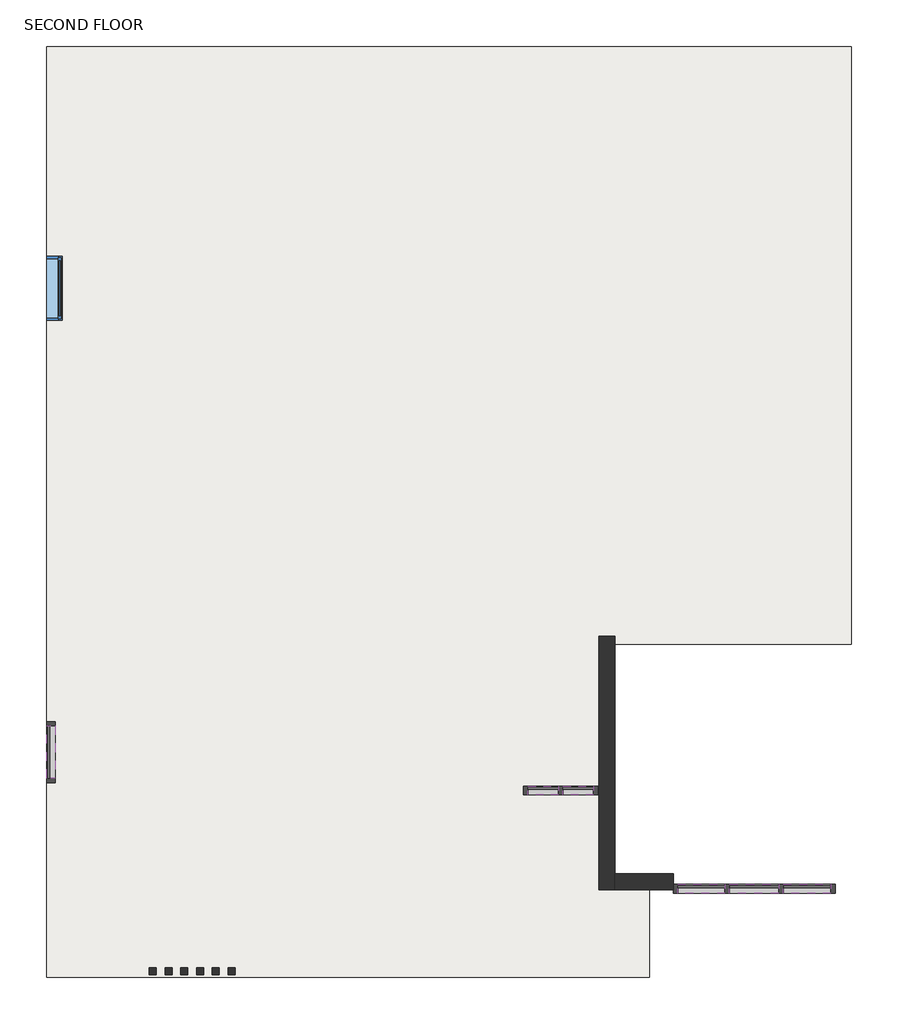
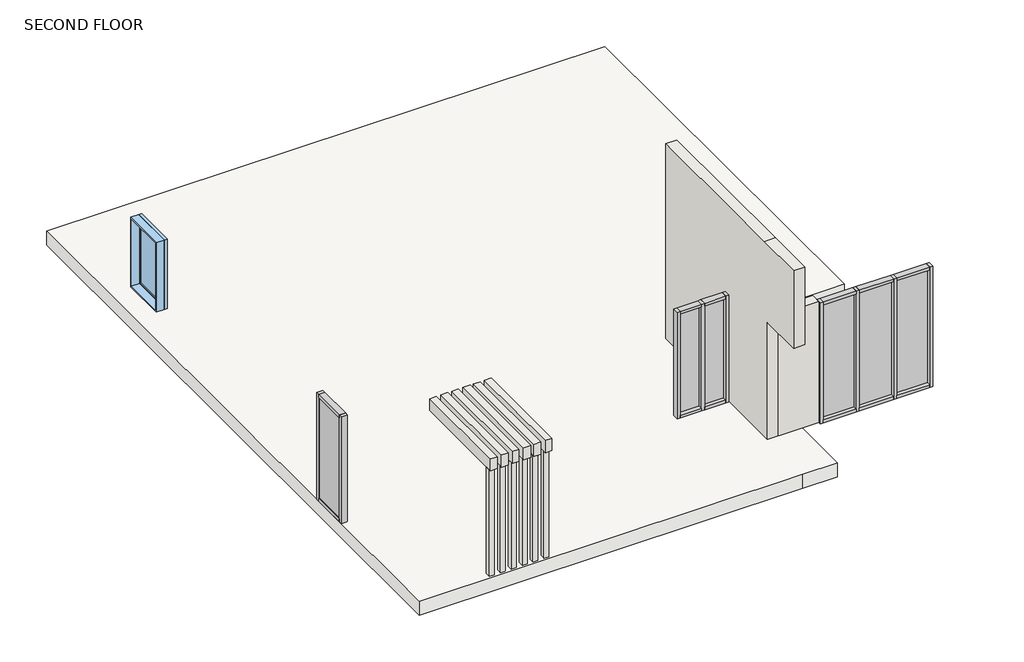
# One storey, incomplete: 21 members, 6 plates, 3 walls, 1 slab, 1 window.
"""IFC4 building model written with IfcOpenShell, lengths in millimetres."""

from ifc_helpers import new_model, si_unit, frame, origin, place, context, project, spatial, polyline, outline, extrude, faceted_brep, transform, mapped, element, save
from components import member_9bbf3b0c, member_f77fa896, member_3f28283e, member_3cbf331d, member_1631f5ff, member_7823a6e7, member_6fb4a552, member_def95f85, system_panel_glazed_aa1e9ff3, system_panel_glazed_6ccdd28e, system_panel_glazed_5a379f96, system_panel_glazed_6abed3b5, walls_2_walls_2_a9f40376, window_cd393ee1

model = new_model("IFC4")

# Units and contexts
model_context = context("Model", 3, world=origin())
ifc_project = project(units=[si_unit("LENGTHUNIT", "METRE", prefix="MILLI")], contexts=[model_context])

# Site, building, storey
site = spatial("IfcSite", under=ifc_project)
building = spatial("IfcBuilding", under=site)
storey = spatial("IfcBuildingStorey", under=building, Name="SECOND FLOOR", Elevation=6096.0)

# Members
placement = place(None, origin())
member_shape = member_9bbf3b0c(model_context)
element("IfcMember", 1, ObjectType="Rectangular Mullion : 2.5\" x 5\" rectangular", at=placement, inside=storey, context=model_context, shape_type="MappedRepresentation", body=[
    mapped(member_shape, transform((94.5792748, 2415.8467494, 6096.0), x_axis=(1.0, 0.0, 0.0), y_axis=(0.0, -1.0, 0.0), z_axis=(0.0, 0.0, -1.0))),
])
element("IfcMember", 2, ObjectType="Rectangular Mullion : 2.5\" x 5\" rectangular", at=placement, inside=storey, context=model_context, shape_type="MappedRepresentation", body=[
    mapped(member_shape, transform((-7754.0425919, 3404.9615229, 6096.0), x_axis=(0.0, 1.0, 0.0), y_axis=(1.0, 0.0, 0.0), z_axis=(0.0, 0.0, -1.0))),
])
element("IfcMember", 3, ObjectType="Rectangular Mullion : 2.5\" x 5\" rectangular", at=placement, inside=storey, context=model_context, shape_type="MappedRepresentation", body=[
    mapped(member_shape, transform((-972.2207252, 2415.8467494, 8432.8), x_axis=(-1.0, 0.0, 0.0), y_axis=(0.0, -1.0, 0.0), z_axis=(0.0, 0.0, 1.0))),
])
element("IfcMember", 4, ObjectType="Rectangular Mullion : 2.5\" x 5\" rectangular", at=placement, inside=storey, context=model_context, shape_type="MappedRepresentation", body=[
    mapped(member_shape, transform((-7754.0425919, 2530.1467494, 8432.8), x_axis=(0.0, -1.0, 0.0), y_axis=(1.0, 0.0, 0.0), z_axis=(0.0, 0.0, 1.0))),
])
member_2_shape = member_f77fa896(model_context)
element("IfcMember", 5, ObjectType="Rectangular Mullion : 2.5\" x 5\" rectangular", at=placement, inside=storey, context=model_context, shape_type="MappedRepresentation", body=[
    mapped(member_2_shape, transform((-7754.0425919, 3341.4615229, 8432.8), x_axis=(0.0, 0.0, 1.0), y_axis=(1.0, 0.0, 0.0), z_axis=(0.0, 1.0, 0.0))),
])
element("IfcMember", 6, ObjectType="Rectangular Mullion : 2.5\" x 5\" rectangular", at=placement, inside=storey, context=model_context, shape_type="MappedRepresentation", body=[
    mapped(member_2_shape, transform((-7754.0425919, 2593.6467494, 6096.0), x_axis=(0.0, 0.0, -1.0), y_axis=(1.0, 0.0, 0.0), z_axis=(0.0, -1.0, 0.0))),
])
member_3_shape = member_3f28283e(model_context)
element("IfcMember", 7, ObjectType="Rectangular Mullion : 2.5\" x 5\" rectangular", at=placement, inside=storey, context=model_context, shape_type="MappedRepresentation", body=[
    mapped(member_3_shape, transform((3498.0918749, 1006.1953049, 6096.0), x_axis=(1.0, 0.0, 0.0), y_axis=(0.0, -1.0, 0.0), z_axis=(0.0, 0.0, -1.0))),
])
element("IfcMember", 8, ObjectType="Rectangular Mullion : 2.5\" x 5\" rectangular", at=placement, inside=storey, context=model_context, shape_type="MappedRepresentation", body=[
    mapped(member_3_shape, transform((1173.991862, 1006.1953049, 8737.6), x_axis=(-1.0, 0.0, 0.0), y_axis=(0.0, -1.0, 0.0), z_axis=(0.0, 0.0, 1.0))),
])
member_4_shape = member_3cbf331d(model_context)
element("IfcMember", 9, ObjectType="Rectangular Mullion : 2.5\" x 5\" rectangular", at=placement, inside=storey, context=model_context, shape_type="MappedRepresentation", body=[
    mapped(member_4_shape, transform((1237.491862, 1006.1953049, 6096.0), x_axis=(0.0, 0.0, -1.0), y_axis=(0.0, -1.0, 0.0), z_axis=(-1.0, 0.0, 0.0))),
])
element("IfcMember", 10, ObjectType="Rectangular Mullion : 2.5\" x 5\" rectangular", at=placement, inside=storey, context=model_context, shape_type="MappedRepresentation", body=[
    mapped(member_4_shape, transform((2755.1418706, 1006.1953049, 6096.0), x_axis=(0.0, 0.0, -1.0), y_axis=(0.0, -1.0, 0.0), z_axis=(-1.0, 0.0, 0.0))),
])
element("IfcMember", 11, ObjectType="Rectangular Mullion : 2.5\" x 5\" rectangular", at=placement, inside=storey, context=model_context, shape_type="MappedRepresentation", body=[
    mapped(member_4_shape, transform((3434.5918749, 1006.1953049, 8737.6), x_axis=(0.0, 0.0, 1.0), y_axis=(0.0, -1.0, 0.0), z_axis=(1.0, 0.0, 0.0))),
])
element("IfcMember", 12, ObjectType="Rectangular Mullion : 2.5\" x 5\" rectangular", at=placement, inside=storey, context=model_context, shape_type="MappedRepresentation", body=[
    mapped(member_4_shape, transform((1916.9418663, 1006.1953049, 8737.6), x_axis=(0.0, 0.0, 1.0), y_axis=(0.0, -1.0, 0.0), z_axis=(1.0, 0.0, 0.0))),
])
member_5_shape = member_1631f5ff(model_context)
element("IfcMember", 13, ObjectType="Rectangular Mullion : 2.5\" x 5\" rectangular", at=placement, inside=storey, context=model_context, shape_type="MappedRepresentation", body=[
    mapped(member_5_shape, transform((1948.6918663, 1006.1953049, 6096.0), x_axis=(1.0, 0.0, 0.0), y_axis=(0.0, -1.0, 0.0), z_axis=(0.0, 0.0, -1.0))),
])
element("IfcMember", 14, ObjectType="Rectangular Mullion : 2.5\" x 5\" rectangular", at=placement, inside=storey, context=model_context, shape_type="MappedRepresentation", body=[
    mapped(member_5_shape, transform((2723.3918706, 1006.1953049, 6096.0), x_axis=(1.0, 0.0, 0.0), y_axis=(0.0, -1.0, 0.0), z_axis=(0.0, 0.0, -1.0))),
])
member_6_shape = member_7823a6e7(model_context)
element("IfcMember", 15, ObjectType="Rectangular Mullion : 2.5\" x 5\" rectangular", at=placement, inside=storey, context=model_context, shape_type="MappedRepresentation", body=[
    mapped(member_6_shape, transform((1980.4418663, 1006.1953049, 6096.0), x_axis=(0.0, 0.0, -1.0), y_axis=(0.0, -1.0, 0.0), z_axis=(-1.0, 0.0, 0.0))),
])
element("IfcMember", 16, ObjectType="Rectangular Mullion : 2.5\" x 5\" rectangular", at=placement, inside=storey, context=model_context, shape_type="MappedRepresentation", body=[
    mapped(member_6_shape, transform((2691.6418706, 1006.1953049, 8737.6), x_axis=(0.0, 0.0, 1.0), y_axis=(0.0, -1.0, 0.0), z_axis=(1.0, 0.0, 0.0))),
])
member_7_shape = member_6fb4a552(model_context)
element("IfcMember", 17, ObjectType="Rectangular Mullion : 2.5\" x 5\" rectangular", at=placement, inside=storey, context=model_context, shape_type="MappedRepresentation", body=[
    mapped(member_7_shape, transform((31.0792748, 2415.8467494, 8432.8), x_axis=(0.0, 0.0, 1.0), y_axis=(0.0, -1.0, 0.0), z_axis=(1.0, 0.0, 0.0))),
])
element("IfcMember", 18, ObjectType="Rectangular Mullion : 2.5\" x 5\" rectangular", at=placement, inside=storey, context=model_context, shape_type="MappedRepresentation", body=[
    mapped(member_7_shape, transform((-470.5707252, 2415.8467494, 8432.8), x_axis=(0.0, 0.0, 1.0), y_axis=(0.0, -1.0, 0.0), z_axis=(1.0, 0.0, 0.0))),
])
element("IfcMember", 19, ObjectType="Rectangular Mullion : 2.5\" x 5\" rectangular", at=placement, inside=storey, context=model_context, shape_type="MappedRepresentation", body=[
    mapped(member_7_shape, transform((-908.7207252, 2415.8467494, 6096.0), x_axis=(0.0, 0.0, -1.0), y_axis=(0.0, -1.0, 0.0), z_axis=(-1.0, 0.0, 0.0))),
])
element("IfcMember", 20, ObjectType="Rectangular Mullion : 2.5\" x 5\" rectangular", at=placement, inside=storey, context=model_context, shape_type="MappedRepresentation", body=[
    mapped(member_7_shape, transform((-407.0707252, 2415.8467494, 6096.0), x_axis=(0.0, 0.0, -1.0), y_axis=(0.0, -1.0, 0.0), z_axis=(-1.0, 0.0, 0.0))),
])
member_8_shape = member_def95f85(model_context)
element("IfcMember", 21, ObjectType="Rectangular Mullion : 2.5\" x 5\" rectangular", at=placement, inside=storey, context=model_context, shape_type="MappedRepresentation", body=[
    mapped(member_8_shape, transform((-438.8207252, 2415.8467494, 6096.0), x_axis=(1.0, 0.0, 0.0), y_axis=(0.0, -1.0, 0.0), z_axis=(0.0, 0.0, -1.0))),
])

# Plates
system_panel_glazed_shape = system_panel_glazed_aa1e9ff3(model_context)
element("IfcPlate", 22, ObjectType="System Panel : Glazed", at=placement, inside=storey, context=model_context, shape_type="MappedRepresentation", body=[
    mapped(system_panel_glazed_shape, transform((-7754.0425919, 2967.5541361, 6159.5), x_axis=(0.0, 1.0, 0.0), y_axis=(-1.0, 0.0, 0.0), z_axis=(0.0, 0.0, 1.0))),
])
system_panel_glazed_2_shape = system_panel_glazed_6ccdd28e(model_context)
element("IfcPlate", 23, ObjectType="System Panel : Glazed", at=placement, inside=storey, context=model_context, shape_type="MappedRepresentation", body=[
    mapped(system_panel_glazed_2_shape, transform((1577.2168642, 1006.1953049, 6159.5), x_axis=(1.0, 0.0, 0.0), y_axis=(0.0, 1.0, 0.0), z_axis=(0.0, 0.0, 1.0))),
])
element("IfcPlate", 24, ObjectType="System Panel : Glazed", at=placement, inside=storey, context=model_context, shape_type="MappedRepresentation", body=[
    mapped(system_panel_glazed_2_shape, transform((3094.8668728, 1006.1953049, 6159.5), x_axis=(1.0, 0.0, 0.0), y_axis=(0.0, 1.0, 0.0), z_axis=(0.0, 0.0, 1.0))),
])
system_panel_glazed_3_shape = system_panel_glazed_5a379f96(model_context)
element("IfcPlate", 25, ObjectType="System Panel : Glazed", at=placement, inside=storey, context=model_context, shape_type="MappedRepresentation", body=[
    mapped(system_panel_glazed_3_shape, transform((2336.0418685, 1006.1953049, 6159.5), x_axis=(1.0, 0.0, 0.0), y_axis=(0.0, 1.0, 0.0), z_axis=(0.0, 0.0, 1.0))),
])
system_panel_glazed_4_shape = system_panel_glazed_6abed3b5(model_context)
element("IfcPlate", 26, ObjectType="System Panel : Glazed", at=placement, inside=storey, context=model_context, shape_type="MappedRepresentation", body=[
    mapped(system_panel_glazed_4_shape, transform((-689.6457252, 2415.8467494, 6159.5), x_axis=(1.0, 0.0, 0.0), y_axis=(0.0, 1.0, 0.0), z_axis=(0.0, 0.0, 1.0))),
])
element("IfcPlate", 27, ObjectType="System Panel : Glazed", at=placement, inside=storey, context=model_context, shape_type="MappedRepresentation", body=[
    mapped(system_panel_glazed_4_shape, transform((-187.9957252, 2415.8467494, 6159.5), x_axis=(1.0, 0.0, 0.0), y_axis=(0.0, 1.0, 0.0), z_axis=(0.0, 0.0, 1.0))),
])

# Slab
element("IfcSlab", 28, ObjectType="Generic - 12\"", at=placement, inside=storey, context=model_context, shape_type="SweptSolid", body=[
    extrude(outline(polyline([(3726.6918749, 13083.8953049), (3726.6918749, 4511.3953049), (107.1918749, 4511.3953049), (107.1918749, 993.4953049), (831.1355684, 993.4953049), (831.1355684, -263.8046951), (108.6382856, -263.8046951), (-7817.6081251, -263.8046951), (-7817.6081251, 13083.8953049), (3726.6918749, 13083.8953049)])), frame((0.0, 0.0, 5791.2), z_axis=(0.0, 0.0, 1.0), x_axis=(1.0, 0.0, 0.0)), (0.0, 0.0, 1.0), 304.8),
])

# Walls
element("IfcWall", 29, ObjectType="9\"", at=placement, inside=storey, context=model_context, shape_type="Brep", body=[
    faceted_brep([(335.8792748, 993.4953049, 6096.0), (335.8792748, 1222.0953049, 6096.0), (335.8792748, 4625.6953049, 6096.0), (335.8792748, 4625.6953049, 10363.2), (335.8792748, 1107.7953049, 10363.2), (335.8792748, 282.2953049, 10363.2), (335.8792748, 53.6953049, 10363.2), (335.8792748, 53.6953049, 8737.6), (335.8792748, 53.6953049, 8661.4), (335.8792748, 993.4953049, 8661.4), (107.2792748, 993.4953049, 6096.0), (107.2792748, 993.4953049, 8661.4), (107.2792748, 53.6953049, 8661.4), (107.2792748, 53.6953049, 10363.2), (107.2792748, 1107.7953049, 10363.2), (107.2792748, 1895.1953049, 10363.2), (107.2792748, 2123.7953049, 10363.2), (107.2792748, 4625.6953049, 10363.2), (107.2792748, 4625.6953049, 6096.0)], [[[0, 1, 2, 3, 4, 5, 6, 7, 8, 9]], [[10, 11, 12, 13, 14, 15, 16, 17, 18]], [[2, 1, 0, 10, 18]], [[3, 2, 18, 17]], [[4, 3, 17, 16, 15, 14]], [[6, 5, 4, 14, 13]], [[8, 7, 6, 13, 12]], [[9, 8, 12, 11]], [[0, 9, 11, 10]]]),
])
element("IfcWall", 30, ObjectType="9\"", at=placement, inside=storey, context=model_context, shape_type="Brep", body=[
    faceted_brep([(335.8792748, 993.4953049, 8737.6), (335.8792748, 993.4953049, 8661.4), (335.8792748, 993.4953049, 6096.0), (1173.991862, 993.4953049, 6096.0), (1173.991862, 993.4953049, 8737.6), (335.8792748, 1222.0953049, 6096.0), (335.8792748, 1222.0953049, 8737.6), (1173.991862, 1222.0953049, 8737.6), (1173.991862, 1222.0953049, 6096.0)], [[[0, 1, 2, 3, 4]], [[5, 6, 7, 8]], [[3, 2, 5, 8]], [[4, 3, 8, 7]], [[0, 4, 7, 6]], [[0, 6, 5, 2, 1]]]),
])
walls_2_walls_2_shape = walls_2_walls_2_a9f40376(model_context)
element("IfcWall", 31, ObjectType="Walls 2 : Walls 2", at=placement, inside=storey, context=model_context, shape_type="MappedRepresentation", body=[
    mapped(walls_2_walls_2_shape, transform((0.0, 0.0, 0.0), x_axis=(1.0, 0.0, 0.0), y_axis=(0.0, 1.0, 0.0), z_axis=(0.0, 0.0, 1.0))),
])

# Window
window_shape = window_cd393ee1(model_context)
element("IfcWindow", 32, ObjectType="Fixed : 36\" x 48\"", at=placement, inside=storey, context=model_context, shape_type="MappedRepresentation", body=[
    mapped(window_shape, transform((-7703.3081251, 9578.6953049, 5791.2), x_axis=(0.0, -1.0, 0.0), y_axis=(1.0, 0.0, 0.0), z_axis=(0.0, 0.0, 1.0))),
])

save(model, "model.ifc")

# Revit data of these elements
# Type "Rectangular Mullion : 2.5\" x 5\" rectangular"
#   built-in parameter 1007304 = 0.416667 (stored number, unit not read)
#   built-in parameter 1007301 = 0.104167 (stored number, unit not read)
#   built-in parameter 1007300 = 0.104167 (stored number, unit not read)
# Type "System Panel : Glazed"
#   Construction Type Id = "GSP4R"
#   Analytic Construction = "1/8 in Pilkington single glazing"
#   Visual Light Transmittance = 0.9
#   Solar Heat Gain Coefficient = 0.86
#   Heat Transfer Coefficient (U) = 1.18115 BTU/(h·ft²·°F)
#   Define Thermal Properties by = 1
# Type "Generic - 12\""
#   Assembly Code = "B1010"
#   Function = 0
#   Layers, outside or top first: 1' - 0" no material (function 1)
# Type "9\""
#   Assembly Code = "B2010"
#   Layers, outside or top first: 0' - 9" "1 wall" (function 1)
# Type "Fixed : 36\" x 48\""
#   Type Mark = "1"
#   Construction Type Id = "GSP4R"
#   Assembly Code = "B2020100"
#   Analytic Construction = "1/8 in Pilkington single glazing"
#   Visual Light Transmittance = 0.9
#   Solar Heat Gain Coefficient = 0.78
#   Heat Transfer Coefficient (U) = 0.6496 BTU/(h·ft²·°F)
#   Height = 5' - 0"
#   Default Sill Height = 3' - 0"
#   Width = 3' - 0"
#   Window Inset = 0' - 0 3/4"
#   Define Thermal Properties by = 1
#   Define Thermal Properties by = 1
#   Glass Pane Material = Glass
#   Sash Material = Sash
#   Wall Closure = (empty or 0)
# Elements 1, 2, 3, 4, 5, 6, 7, 8, 9, 10, 11, 12, 13, 14, 15, 16, 17, 18, 19, 20, 21 (IfcMember, "Rectangular Mullion : 2.5\" x 5\" rectangular")
#   Phase Created = New Construction
#   Materials on its faces: "Aluminum"
# Elements 22, 23, 24, 25, 26, 27 (IfcPlate, "System Panel : Glazed")
#   Phase Created = New Construction
#   Materials on its faces: "Glass"
# Element 28 (IfcSlab, "Generic - 12\"")
#   Height Offset From Level = 0' - 0"
#   Phase Created = New Construction
#   Materials on its faces: "Acoustic Ceiling Tile 24 x 24", "Default Floor", "1 white"
# Element 29 (IfcWall, "9\"")
#   Top Offset = 0' - 0"
#   Base Offset = 0' - 0"
#   wall height = 14' - 0"
#   Phase Created = New Construction
#   Base Constraint = SECOND FLOOR
#   Top Constraint = SLAB 2
#   Materials on its faces: "1 wall"
# Element 30 (IfcWall, "9\"")
#   Top Offset = 0' - 0"
#   Base Offset = 0' - 0"
#   Unconnected Height = 8' - 8"
#   wall height = 8' - 8"
#   Phase Created = New Construction
#   Base Constraint = SECOND FLOOR
#   Materials on its faces: "1 wall"
# Element 31 (IfcWall, "Walls 2 : Walls 2")
#   Phase Created = New Construction
#   Materials on its faces: "1 white", "Default Wall"
# Element 32 (IfcWindow, "Fixed : 36\" x 48\"")
#   Mark = "3"
#   Phase Created = New Construction
#   Materials on its faces: "Sash", "Glass"
# Materials
#   "1 wall": class "Generic", colour RGB 172 157 136, transparency 0, Cost = 0
#   "Glass": class "Glass", colour RGB 0 128 192, transparency 0.75, Description = "Soda Lime Glass", Cost = 0
#   "Sash": class "Wood", colour RGB 224 178 126, transparency 0, Cost = 0
#   "Aluminum": class "Metal", colour RGB 247 247 247, transparency 0, Description = "Aluminum 6061", Cost = 0
#   "Acoustic Ceiling Tile 24 x 24": class "Generic", colour RGB 232 232 232, transparency 0, Description = "Acoustic Ceiling Tile 24 x 24", Cost = 0
#   "Default Floor": colour RGB 128 128 128, transparency 0, Cost = 0
#   "1 white": class "Generic", colour RGB 244 245 241, transparency 0, Cost = 0
#   "Default Wall": colour RGB 128 128 128, transparency 0, Cost = 0
